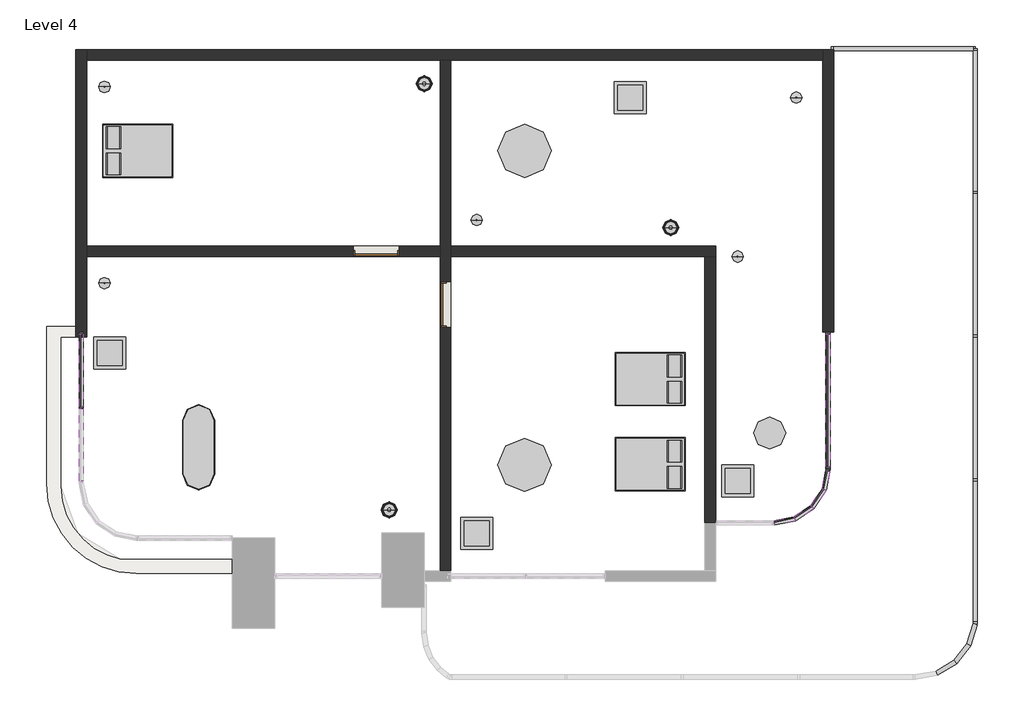
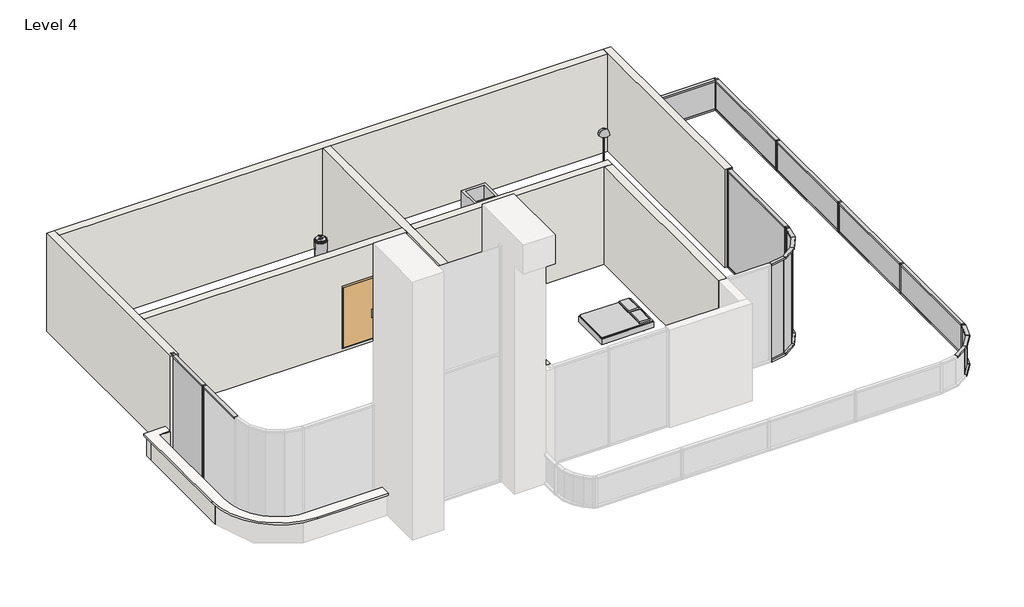
# One storey, part 2 of 2: 40 members, 13 plates, 9 walls, 7 furniture elements, 7 light fixtures, 4 geographic elements, 3 proxies, 2 doors, 1 slab.
"""IFC4 building model written with IfcOpenShell, lengths in millimetres."""

from ifc_helpers import new_model, si_unit, point, frame, frame_2d, origin, place, context, project, spatial, polyline, circle_curve, trimmed, segment, composite_curve, outline, extrude, faceted_brep, transform, mapped, element, save
from components import recycle_bin_round_recycle_bin_round_6e7ed866, door_bb6275b8, furniture_1d2926bd, furniture_e05f6f82, furniture_720490b2, furniture_905aceb5, geographic_element_4c884dac, floor_lamp_hemispheric_100w_120v_bd9db648, table_lamp_standard_100w_120v_6e8cd8b1, member_e5c989f4, member_5be86ab4, member_2115025b, member_820ab859, member_6051e8ad, member_ad26f02d, member_4ff03cd1, member_efc2c738, member_55924089, member_20b53a5f, member_9703a30f, member_ec2bec36, member_2b49869a, member_75074519, member_fe018dc2, member_83685764, member_73d0c9ee, system_panel_glazed_319e86f2, system_panel_glazed_5d8041e7, system_panel_glazed_56e4e121, system_panel_glazed_16a45962, system_panel_glazed_93b9a344, system_panel_glazed_b0cc1a2f, system_panel_glazed_8d4a2524, system_panel_glazed_b9e36109

model = new_model("IFC4")

# Units and contexts
model_context = context("Model", 3, world=origin())
ifc_project = project(units=[si_unit("LENGTHUNIT", "METRE", prefix="MILLI")], contexts=[model_context])

# Site, building, storey
site = spatial("IfcSite", under=ifc_project)
building = spatial("IfcBuilding", under=site)
storey = spatial("IfcBuildingStorey", under=building, Name="Level 4", Elevation=6096.0)

# Proxies
placement = place(None, origin())
recycle_bin_round_recycle_bin_round_shape = recycle_bin_round_recycle_bin_round_6e7ed866(model_context)
element("IfcBuildingElementProxy", 1, Name="Recycle Bin-Round : Recycle Bin-Round", ObjectType="Recycle Bin-Round : Recycle Bin-Round", at=placement, inside=storey, context=model_context, shape_type="MappedRepresentation", body=[
    mapped(recycle_bin_round_recycle_bin_round_shape, transform((-7920.936879, -2221.8562261, 6096.0), x_axis=(1.0, 0.0, 0.0), y_axis=(0.0, 1.0, 0.0), z_axis=(0.0, 0.0, 1.0))),
])
element("IfcBuildingElementProxy", 2, Name="Recycle Bin-Round : Recycle Bin-Round", ObjectType="Recycle Bin-Round : Recycle Bin-Round", at=placement, inside=storey, context=model_context, shape_type="MappedRepresentation", body=[
    mapped(recycle_bin_round_recycle_bin_round_shape, transform((-6917.636879, 9970.1437739, 6096.0), x_axis=(1.0, 0.0, 0.0), y_axis=(0.0, 1.0, 0.0), z_axis=(0.0, 0.0, 1.0))),
])
element("IfcBuildingElementProxy", 3, Name="Recycle Bin-Round : Recycle Bin-Round", ObjectType="Recycle Bin-Round : Recycle Bin-Round", at=placement, inside=storey, context=model_context, shape_type="MappedRepresentation", body=[
    mapped(recycle_bin_round_recycle_bin_round_shape, transform((130.863121, 5855.3437739, 6096.0), x_axis=(1.0, 0.0, 0.0), y_axis=(0.0, 1.0, 0.0), z_axis=(0.0, 0.0, 1.0))),
])

# Doors
door_shape = door_bb6275b8(model_context)
element("IfcDoor", 4, ObjectType="Door-Passage-Single-Flush-Dbl_Acting : 48\" x 96\"", at=placement, inside=storey, context=model_context, shape_type="MappedRepresentation", body=[
    mapped(door_shape, transform((-8289.236879, 5183.9591958, 6096.0), x_axis=(-1.0, 0.0, 0.0), y_axis=(0.0, -1.0, 0.0), z_axis=(0.0, 0.0, 1.0))),
])
element("IfcDoor", 5, ObjectType="Door-Passage-Single-Flush-Dbl_Acting : 48\" x 96\"", at=placement, inside=storey, context=model_context, shape_type="MappedRepresentation", body=[
    mapped(door_shape, transform((-6301.686879, 3653.6091958, 6096.0), x_axis=(0.0, 1.0, 0.0), y_axis=(-1.0, 0.0, 0.0), z_axis=(0.0, 0.0, 1.0))),
])

# Furniture
furniture_shape = furniture_1d2926bd(model_context)
element("IfcFurniture", 6, ObjectType="Bed-Box : Queen 60\" x 79\"", at=placement, inside=storey, context=model_context, shape_type="MappedRepresentation", body=[
    mapped(furniture_shape, transform((-15345.945017, 7713.2913149, 6096.0), x_axis=(0.0, 1.0000000000000002, 0.0), y_axis=(-1.0000000000000002, 0.0, 0.0), z_axis=(0.0, 0.0, 1.0))),
])
element("IfcFurniture", 7, ObjectType="Bed-Box : Queen 60\" x 79\"", at=placement, inside=storey, context=model_context, shape_type="MappedRepresentation", body=[
    mapped(furniture_shape, transform((-218.9073708, -579.2383452, 6096.0), x_axis=(0.0, -1.0, 0.0), y_axis=(1.0, 0.0, 0.0), z_axis=(0.0, 0.0, 1.0))),
])
element("IfcFurniture", 8, ObjectType="Bed-Box : Queen 60\" x 79\"", at=placement, inside=storey, context=model_context, shape_type="MappedRepresentation", body=[
    mapped(furniture_shape, transform((-218.9073708, 1859.1616548, 6096.0), x_axis=(0.0, -1.0, 0.0), y_axis=(1.0, 0.0, 0.0), z_axis=(0.0, 0.0, 1.0))),
])
furniture_2_shape = furniture_e05f6f82(model_context)
element("IfcFurniture", 9, ObjectType="Table-Dining Oval : 36\" x 96\" Glass Top", at=placement, inside=storey, context=model_context, shape_type="MappedRepresentation", body=[
    mapped(furniture_2_shape, transform((-13727.1545191, -29.9659461, 6096.0), x_axis=(0.0, 1.0000000000000002, 0.0), y_axis=(-1.0000000000000002, 0.0, 0.0), z_axis=(0.0, 0.0, 1.0))),
])
furniture_3_shape = furniture_720490b2(model_context)
element("IfcFurniture", 10, ObjectType="Table-Dining Round : 60\" Diameter", at=placement, inside=storey, context=model_context, shape_type="MappedRepresentation", body=[
    mapped(furniture_3_shape, transform((-4151.1188462, -754.2775376, 6096.0), x_axis=(1.0, 0.0, 0.0), y_axis=(0.0, 1.0, 0.0), z_axis=(0.0, 0.0, 1.0))),
])
element("IfcFurniture", 11, ObjectType="Table-Dining Round : 60\" Diameter", at=placement, inside=storey, context=model_context, shape_type="MappedRepresentation", body=[
    mapped(furniture_3_shape, transform((-4151.1188462, 8237.3224624, 6096.0), x_axis=(1.0, 0.0, 0.0), y_axis=(0.0, 1.0, 0.0), z_axis=(0.0, 0.0, 1.0))),
])
furniture_4_shape = furniture_905aceb5(model_context)
element("IfcFurniture", 12, ObjectType="Table-Dining Round w Chairs : 36\" Diameter", at=placement, inside=storey, context=model_context, shape_type="MappedRepresentation", body=[
    mapped(furniture_4_shape, transform((2855.1330373, 160.1224624, 6096.0), x_axis=(1.0, 0.0, 0.0), y_axis=(0.0, 1.0, 0.0), z_axis=(0.0, 0.0, 1.0))),
])

# Geographic elements
geographic_element_shape = geographic_element_4c884dac(model_context)
element("IfcGeographicElement", 13, ObjectType="Planter : 36\" x 36\"", at=placement, inside=storey, context=model_context, shape_type="MappedRepresentation", body=[
    mapped(geographic_element_shape, transform((2044.4150045, -1396.3562261, 6096.0), x_axis=(1.0, 0.0, 0.0), y_axis=(0.0, 1.0, 0.0), z_axis=(0.0, 0.0, 1.0))),
])
element("IfcGeographicElement", 14, ObjectType="Planter : 36\" x 36\"", at=placement, inside=storey, context=model_context, shape_type="MappedRepresentation", body=[
    mapped(geographic_element_shape, transform((-5419.036879, -2899.5908042, 6096.0), x_axis=(1.0, 0.0, 0.0), y_axis=(0.0, 1.0, 0.0), z_axis=(0.0, 0.0, 1.0))),
])
element("IfcGeographicElement", 15, ObjectType="Planter : 36\" x 36\"", at=placement, inside=storey, context=model_context, shape_type="MappedRepresentation", body=[
    mapped(geographic_element_shape, transform((-15909.236879, 2261.2437739, 6096.0), x_axis=(1.0, 0.0, 0.0), y_axis=(0.0, 1.0, 0.0), z_axis=(0.0, 0.0, 1.0))),
])
element("IfcGeographicElement", 16, ObjectType="Planter : 36\" x 36\"", at=placement, inside=storey, context=model_context, shape_type="MappedRepresentation", body=[
    mapped(geographic_element_shape, transform((-1024.836879, 9576.4437739, 6096.0), x_axis=(1.0, 0.0, 0.0), y_axis=(0.0, 1.0, 0.0), z_axis=(0.0, 0.0, 1.0))),
])

# Light fixtures
floor_lamp_hemispheric_100w_120v_shape = floor_lamp_hemispheric_100w_120v_bd9db648(model_context)
element("IfcLightFixture", 17, ObjectType="Floor Lamp - Hemispheric : 100W - 120V", at=placement, inside=storey, context=model_context, shape_type="MappedRepresentation", body=[
    mapped(floor_lamp_hemispheric_100w_120v_shape, transform((-16061.636879, 4263.2091958, 6096.0), x_axis=(1.0, 0.0, 0.0), y_axis=(0.0, 1.0, 0.0), z_axis=(0.0, 0.0, 1.0))),
])
element("IfcLightFixture", 18, ObjectType="Floor Lamp - Hemispheric : 100W - 120V", at=placement, inside=storey, context=model_context, shape_type="MappedRepresentation", body=[
    mapped(floor_lamp_hemispheric_100w_120v_shape, transform((-16061.636879, 9881.2437739, 6096.0), x_axis=(1.0, 0.0, 0.0), y_axis=(0.0, 1.0, 0.0), z_axis=(0.0, 0.0, 1.0))),
])
element("IfcLightFixture", 19, ObjectType="Floor Lamp - Hemispheric : 100W - 120V", at=placement, inside=storey, context=model_context, shape_type="MappedRepresentation", body=[
    mapped(floor_lamp_hemispheric_100w_120v_shape, transform((3720.8150045, 9576.4437739, 6096.0), x_axis=(1.0, 0.0, 0.0), y_axis=(0.0, 1.0, 0.0), z_axis=(0.0, 0.0, 1.0))),
])
element("IfcLightFixture", 20, ObjectType="Floor Lamp - Hemispheric : 100W - 120V", at=placement, inside=storey, context=model_context, shape_type="MappedRepresentation", body=[
    mapped(floor_lamp_hemispheric_100w_120v_shape, transform((2044.4150045, 5025.2091958, 6096.0), x_axis=(1.0, 0.0, 0.0), y_axis=(0.0, 1.0, 0.0), z_axis=(0.0, 0.0, 1.0))),
])
element("IfcLightFixture", 21, ObjectType="Floor Lamp - Hemispheric : 100W - 120V", at=placement, inside=storey, context=model_context, shape_type="MappedRepresentation", body=[
    mapped(floor_lamp_hemispheric_100w_120v_shape, transform((-5419.036879, 6071.2437739, 6096.0), x_axis=(1.0, 0.0, 0.0), y_axis=(0.0, 1.0, 0.0), z_axis=(0.0, 0.0, 1.0))),
])
table_lamp_standard_100w_120v_shape = table_lamp_standard_100w_120v_6e8cd8b1(model_context)
element("IfcLightFixture", 22, ObjectType="Table Lamp - Standard : 100W - 120V", at=placement, inside=storey, context=model_context, shape_type="MappedRepresentation", body=[
    mapped(table_lamp_standard_100w_120v_shape, transform((-4047.436879, -939.1562261, 6096.0), x_axis=(1.0, 0.0, 0.0), y_axis=(0.0, 1.0, 0.0), z_axis=(0.0, 0.0, 1.0))),
])
element("IfcLightFixture", 23, ObjectType="Table Lamp - Standard : 100W - 120V", at=placement, inside=storey, context=model_context, shape_type="MappedRepresentation", body=[
    mapped(table_lamp_standard_100w_120v_shape, transform((-4047.436879, 8052.4437739, 6096.0), x_axis=(1.0, 0.0, 0.0), y_axis=(0.0, 1.0, 0.0), z_axis=(0.0, 0.0, 1.0))),
])

# Members
member_shape = member_e5c989f4(model_context)
element("IfcMember", 24, ObjectType="Rectangular Mullion : 2.5\" x 5\" rectangular", at=placement, inside=storey, context=model_context, shape_type="MappedRepresentation", body=[
    mapped(member_shape, transform((-16724.4155088, 709.8310564, 5994.4), x_axis=(0.0, 1.0, 0.0), y_axis=(1.0, 0.0, 0.0), z_axis=(0.0, 0.0, -1.0))),
])
member_2_shape = member_5be86ab4(model_context)
element("IfcMember", 25, ObjectType="Rectangular Mullion : 2.5\" x 5\" rectangular", at=placement, inside=storey, context=model_context, shape_type="MappedRepresentation", body=[
    mapped(member_2_shape, transform((4635.2150045, -1049.5389207, 5994.4), x_axis=(0.19509032201613002, 0.9807852804032301, 0.0), y_axis=(0.9807852804032301, -0.19509032201613002, 0.0), z_axis=(0.0, 0.0, -1.0))),
])
element("IfcMember", 26, ObjectType="Rectangular Mullion : 2.5\" x 5\" rectangular", at=placement, inside=storey, context=model_context, shape_type="MappedRepresentation", body=[
    mapped(member_2_shape, transform((4635.2150045, 2870.8437739, 5994.4), x_axis=(0.0, 1.0, 0.0), y_axis=(1.0, 0.0, 0.0), z_axis=(0.0, 0.0, -1.0))),
])
element("IfcMember", 27, ObjectType="Rectangular Mullion : 2.5\" x 5\" rectangular", at=placement, inside=storey, context=model_context, shape_type="MappedRepresentation", body=[
    mapped(member_2_shape, transform((-16724.4155088, 2870.8437739, 5994.4), x_axis=(0.0, 1.0, 0.0), y_axis=(1.0, 0.0, 0.0), z_axis=(0.0, 0.0, -1.0))),
])
element("IfcMember", 28, ObjectType="Rectangular Mullion : 2.5\" x 5\" rectangular", at=placement, inside=storey, context=model_context, shape_type="MappedRepresentation", body=[
    mapped(member_2_shape, transform((4635.2150045, -1049.5389207, 9956.8), x_axis=(0.0, -1.0, 0.0), y_axis=(1.0, 0.0, 0.0), z_axis=(0.0, 0.0, 1.0))),
])
member_3_shape = member_2115025b(model_context)
element("IfcMember", 29, ObjectType="Rectangular Mullion : 2.5\" x 5\" rectangular", at=placement, inside=storey, context=model_context, shape_type="MappedRepresentation", body=[
    mapped(member_3_shape, transform((4635.2150045, 2807.3437739, 9956.8), x_axis=(0.0, 0.0, 1.0), y_axis=(1.0, 0.0, 0.0), z_axis=(0.0, 1.0, 0.0))),
])
element("IfcMember", 30, ObjectType="Rectangular Mullion : 2.5\" x 5\" rectangular", at=placement, inside=storey, context=model_context, shape_type="MappedRepresentation", body=[
    mapped(member_3_shape, transform((4635.2150045, -986.0389207, 5994.4), x_axis=(0.0, 0.0, -1.0), y_axis=(1.0, 0.0, 0.0), z_axis=(0.0, -1.0, 0.0))),
])
member_4_shape = member_820ab859(model_context)
element("IfcMember", 31, ObjectType="Rectangular Mullion : 2.5\" x 5\" rectangular", at=placement, inside=storey, context=model_context, shape_type="MappedRepresentation", body=[
    mapped(member_4_shape, transform((-16724.4155088, 2807.3437739, 9956.8), x_axis=(0.0, 0.0, 1.0), y_axis=(1.0, 0.0, 0.0), z_axis=(0.0, 1.0, 0.0))),
])
element("IfcMember", 32, ObjectType="Rectangular Mullion : 2.5\" x 5\" rectangular", at=placement, inside=storey, context=model_context, shape_type="MappedRepresentation", body=[
    mapped(member_4_shape, transform((-16724.4155088, 678.0810564, 9956.8), x_axis=(0.0, 0.0, 1.0), y_axis=(1.0, 0.0, 0.0), z_axis=(0.0, 1.0, 0.0))),
])
element("IfcMember", 33, ObjectType="Rectangular Mullion : 2.5\" x 5\" rectangular", at=placement, inside=storey, context=model_context, shape_type="MappedRepresentation", body=[
    mapped(member_4_shape, transform((-16724.4155088, 741.5810564, 5994.4), x_axis=(0.0, 0.0, -1.0), y_axis=(1.0, 0.0, 0.0), z_axis=(0.0, -1.0, 0.0))),
])
member_5_shape = member_6051e8ad(model_context)
element("IfcMember", 34, ObjectType="Rectangular Mullion : 2.5\" x 5\" rectangular", at=placement, inside=storey, context=model_context, shape_type="MappedRepresentation", body=[
    mapped(member_5_shape, transform((3089.963121, -2594.7908042, 5994.4), x_axis=(0.0, 0.0, -1.0), y_axis=(0.19509032201612592, -0.9807852804032309, 0.0), z_axis=(-0.9807852804032309, -0.19509032201612592, 0.0))),
])
member_6_shape = member_ad26f02d(model_context)
element("IfcMember", 35, ObjectType="Rectangular Mullion : 2.5\" x 5\" rectangular", at=placement, inside=storey, context=model_context, shape_type="MappedRepresentation", body=[
    mapped(member_6_shape, transform((3681.3054157, -2477.1655084, 9956.8), x_axis=(0.0, 0.0, 1.0), y_axis=(0.19509032201612592, -0.9807852804032309, 0.0), z_axis=(0.9807852804032309, 0.19509032201612592, 0.0))),
])
member_7_shape = member_4ff03cd1(model_context)
element("IfcMember", 36, ObjectType="Rectangular Mullion : 2.5\" x 5\" rectangular", at=placement, inside=storey, context=model_context, shape_type="MappedRepresentation", body=[
    mapped(member_7_shape, transform((4182.6212065, -2142.1970062, 9956.8), x_axis=(0.0, 0.0, 1.0), y_axis=(0.5555702330196008, -0.8314696123025462, 0.0), z_axis=(0.8314696123025462, 0.5555702330196008, 0.0))),
])
element("IfcMember", 37, ObjectType="Rectangular Mullion : 2.5\" x 5\" rectangular", at=placement, inside=storey, context=model_context, shape_type="MappedRepresentation", body=[
    mapped(member_7_shape, transform((3681.3054157, -2477.1655084, 5994.4), x_axis=(0.0, 0.0, -1.0), y_axis=(0.5555702330196008, -0.8314696123025462, 0.0), z_axis=(-0.8314696123025462, -0.5555702330196008, 0.0))),
])
member_8_shape = member_efc2c738(model_context)
element("IfcMember", 38, ObjectType="Rectangular Mullion : 2.5\" x 5\" rectangular", at=placement, inside=storey, context=model_context, shape_type="MappedRepresentation", body=[
    mapped(member_8_shape, transform((4622.826769, -1111.818786, 9956.8), x_axis=(0.0, 0.0, 1.0), y_axis=(0.9807852804032301, -0.19509032201613, 0.0), z_axis=(0.19509032201612997, 0.98078528040323, 0.0))),
])
element("IfcMember", 39, ObjectType="Rectangular Mullion : 2.5\" x 5\" rectangular", at=placement, inside=storey, context=model_context, shape_type="MappedRepresentation", body=[
    mapped(member_7_shape, transform((4182.6212065, -2142.1970062, 5994.4), x_axis=(0.0, 0.0, -1.0), y_axis=(0.831469612302544, -0.5555702330196041, 0.0), z_axis=(-0.5555702330196041, -0.831469612302544, 0.0))),
])
element("IfcMember", 40, ObjectType="Rectangular Mullion : 2.5\" x 5\" rectangular", at=placement, inside=storey, context=model_context, shape_type="MappedRepresentation", body=[
    mapped(member_7_shape, transform((4517.5897087, -1640.8812154, 9956.8), x_axis=(0.0, 0.0, 1.0), y_axis=(0.831469612302544, -0.5555702330196041, 0.0), z_axis=(0.5555702330196041, 0.831469612302544, 0.0))),
])
member_9_shape = member_55924089(model_context)
element("IfcMember", 41, ObjectType="Rectangular Mullion : 2.5\" x 5\" rectangular", at=placement, inside=storey, context=model_context, shape_type="MappedRepresentation", body=[
    mapped(member_9_shape, transform((4517.5897087, -1640.8812154, 5994.4), x_axis=(0.0, 0.0, -1.0), y_axis=(0.9807852804032301, -0.19509032201613008, 0.0), z_axis=(-0.19509032201613008, -0.9807852804032301, 0.0))),
])
member_10_shape = member_20b53a5f(model_context)
element("IfcMember", 42, ObjectType="Rectangular Mullion : 2.5\" x 5\" rectangular", at=placement, inside=storey, context=model_context, shape_type="MappedRepresentation", body=[
    mapped(member_10_shape, transform((8839.2, 10909.3, 7213.6), x_axis=(0.0, 0.0, 1.0), y_axis=(1.0, 0.0, 0.0), z_axis=(0.0, 1.0, 0.0))),
])
element("IfcMember", 43, ObjectType="Rectangular Mullion : 2.5\" x 5\" rectangular", at=placement, inside=storey, context=model_context, shape_type="MappedRepresentation", body=[
    mapped(member_10_shape, transform((8839.2, -1403.35, 7213.6), x_axis=(0.0, 0.0, 1.0), y_axis=(1.0, 0.0, 0.0), z_axis=(0.0, 1.0, 0.0))),
])
member_11_shape = member_9703a30f(model_context)
element("IfcMember", 44, ObjectType="Rectangular Mullion : 2.5\" x 5\" rectangular", at=placement, inside=storey, context=model_context, shape_type="MappedRepresentation", body=[
    mapped(member_11_shape, transform((8839.2, 2711.45, 7213.6), x_axis=(0.0, 0.0, 1.0), y_axis=(1.0, 0.0, 0.0), z_axis=(0.0, 1.0, 0.0))),
])
element("IfcMember", 45, ObjectType="Rectangular Mullion : 2.5\" x 5\" rectangular", at=placement, inside=storey, context=model_context, shape_type="MappedRepresentation", body=[
    mapped(member_11_shape, transform((8839.2, 6826.25, 7213.6), x_axis=(0.0, 0.0, 1.0), y_axis=(1.0, 0.0, 0.0), z_axis=(0.0, 1.0, 0.0))),
])
element("IfcMember", 46, ObjectType="Rectangular Mullion : 2.5\" x 5\" rectangular", at=placement, inside=storey, context=model_context, shape_type="MappedRepresentation", body=[
    mapped(member_10_shape, transform((8839.2, -5422.9, 5994.4), x_axis=(0.0, 0.0, -1.0), y_axis=(1.0, 0.0, 0.0), z_axis=(0.0, -1.0, 0.0))),
])
element("IfcMember", 47, ObjectType="Rectangular Mullion : 2.5\" x 5\" rectangular", at=placement, inside=storey, context=model_context, shape_type="MappedRepresentation", body=[
    mapped(member_10_shape, transform((8839.2, 6889.75, 5994.4), x_axis=(0.0, 0.0, -1.0), y_axis=(1.0, 0.0, 0.0), z_axis=(0.0, -1.0, 0.0))),
])
element("IfcMember", 48, ObjectType="Rectangular Mullion : 2.5\" x 5\" rectangular", at=placement, inside=storey, context=model_context, shape_type="MappedRepresentation", body=[
    mapped(member_11_shape, transform((8839.2, -1339.85, 5994.4), x_axis=(0.0, 0.0, -1.0), y_axis=(1.0, 0.0, 0.0), z_axis=(0.0, -1.0, 0.0))),
])
element("IfcMember", 49, ObjectType="Rectangular Mullion : 2.5\" x 5\" rectangular", at=placement, inside=storey, context=model_context, shape_type="MappedRepresentation", body=[
    mapped(member_11_shape, transform((8839.2, 2774.95, 5994.4), x_axis=(0.0, 0.0, -1.0), y_axis=(1.0, 0.0, 0.0), z_axis=(0.0, -1.0, 0.0))),
])
member_12_shape = member_ec2bec36(model_context)
element("IfcMember", 50, ObjectType="Rectangular Mullion : 2.5\" x 5\" rectangular", at=placement, inside=storey, context=model_context, shape_type="MappedRepresentation", body=[
    mapped(member_12_shape, transform((4787.9, 10972.8, 7213.6), x_axis=(0.0, 0.0, 1.0), y_axis=(0.0, 1.0, 0.0), z_axis=(-1.0, 0.0, 0.0))),
])
element("IfcMember", 51, ObjectType="Rectangular Mullion : 2.5\" x 5\" rectangular", at=placement, inside=storey, context=model_context, shape_type="MappedRepresentation", body=[
    mapped(member_12_shape, transform((8775.7, 10972.8, 5994.4), x_axis=(0.0, 0.0, -1.0), y_axis=(0.0, 1.0, 0.0), z_axis=(1.0, 0.0, 0.0))),
])
member_13_shape = member_2b49869a(model_context)
element("IfcMember", 52, ObjectType="Rectangular Mullion : 2.5\" x 5\" rectangular", at=placement, inside=storey, context=model_context, shape_type="MappedRepresentation", body=[
    mapped(member_13_shape, transform((8839.2, -1371.6, 5994.4), x_axis=(0.0, 1.0, 0.0), y_axis=(1.0, 0.0, 0.0), z_axis=(0.0, 0.0, -1.0))),
])
element("IfcMember", 53, ObjectType="Rectangular Mullion : 2.5\" x 5\" rectangular", at=placement, inside=storey, context=model_context, shape_type="MappedRepresentation", body=[
    mapped(member_13_shape, transform((8839.2, 2743.2, 5994.4), x_axis=(0.0, 1.0, 0.0), y_axis=(1.0, 0.0, 0.0), z_axis=(0.0, 0.0, -1.0))),
])
element("IfcMember", 54, ObjectType="Rectangular Mullion : 2.5\" x 5\" rectangular", at=placement, inside=storey, context=model_context, shape_type="MappedRepresentation", body=[
    mapped(member_13_shape, transform((8839.2, 6858.0, 5994.4), x_axis=(0.0, 1.0, 0.0), y_axis=(1.0, 0.0, 0.0), z_axis=(0.0, 0.0, -1.0))),
])
member_14_shape = member_75074519(model_context)
element("IfcMember", 55, ObjectType="Rectangular Mullion : 2.5\" x 5\" rectangular", at=placement, inside=storey, context=model_context, shape_type="MappedRepresentation", body=[
    mapped(member_14_shape, transform((8839.2, 10972.8, 5994.4), x_axis=(0.0, 1.0, 0.0), y_axis=(1.0, 0.0, 0.0), z_axis=(0.0, 0.0, -1.0))),
])
element("IfcMember", 56, ObjectType="Rectangular Mullion : 2.5\" x 5\" rectangular", at=placement, inside=storey, context=model_context, shape_type="MappedRepresentation", body=[
    mapped(member_14_shape, transform((4724.4, 10972.8, 5994.4), x_axis=(-1.0, 0.0, 0.0), y_axis=(0.0, 1.0, 0.0), z_axis=(0.0, 0.0, -1.0))),
])
element("IfcMember", 57, ObjectType="Rectangular Mullion : 2.5\" x 5\" rectangular", at=placement, inside=storey, context=model_context, shape_type="MappedRepresentation", body=[
    mapped(member_14_shape, transform((8839.2, -5486.4, 7213.6), x_axis=(0.0, -1.0, 0.0), y_axis=(1.0, 0.0, 0.0), z_axis=(0.0, 0.0, 1.0))),
])
element("IfcMember", 58, ObjectType="Rectangular Mullion : 2.5\" x 5\" rectangular", at=placement, inside=storey, context=model_context, shape_type="MappedRepresentation", body=[
    mapped(member_14_shape, transform((8839.2, 10972.8, 7213.6), x_axis=(1.0, 0.0, 0.0), y_axis=(0.0, 1.0, 0.0), z_axis=(0.0, 0.0, 1.0))),
])
member_15_shape = member_fe018dc2(model_context)
element("IfcMember", 59, ObjectType="Rectangular Mullion : 2.5\" x 5\" rectangular", at=placement, inside=storey, context=model_context, shape_type="MappedRepresentation", body=[
    mapped(member_15_shape, transform((8263.7156594, -6574.9310806, 5994.4), x_axis=(0.0, 0.0, -1.0), y_axis=(0.7856364667820415, -0.6186884046612077, 0.0), z_axis=(-0.6186884046612077, -0.7856364667820415, 0.0))),
])
element("IfcMember", 60, ObjectType="Rectangular Mullion : 2.5\" x 5\" rectangular", at=placement, inside=storey, context=model_context, shape_type="MappedRepresentation", body=[
    mapped(member_15_shape, transform((8650.9164441, -6083.2472958, 7213.6), x_axis=(0.0, 0.0, 1.0), y_axis=(0.7856364667820415, -0.6186884046612077, 0.0), z_axis=(0.6186884046612077, 0.7856364667820415, 0.0))),
])
element("IfcMember", 61, ObjectType="Rectangular Mullion : 2.5\" x 5\" rectangular", at=placement, inside=storey, context=model_context, shape_type="MappedRepresentation", body=[
    mapped(member_15_shape, transform((8263.7156594, -6574.9310806, 7213.6), x_axis=(0.0, 0.0, 1.0), y_axis=(0.5160512694614295, -0.856557696414694, 0.0), z_axis=(0.8565576964146939, 0.5160512694614294, 0.0))),
])
member_16_shape = member_83685764(model_context)
element("IfcMember", 62, ObjectType="Rectangular Mullion : 2.5\" x 5\" rectangular", at=placement, inside=storey, context=model_context, shape_type="MappedRepresentation", body=[
    mapped(member_16_shape, transform((8839.2, -5486.4, 7213.6), x_axis=(0.0, 0.0, 1.0), y_axis=(0.9536718825126238, -0.30084870035422845, 0.0), z_axis=(0.30084870035422845, 0.9536718825126238, 0.0))),
])
member_17_shape = member_73d0c9ee(model_context)
element("IfcMember", 63, ObjectType="Rectangular Mullion : 2.5\" x 5\" rectangular", at=placement, inside=storey, context=model_context, shape_type="MappedRepresentation", body=[
    mapped(member_17_shape, transform((8650.9164441, -6083.2472958, 5994.4), x_axis=(0.0, 0.0, -1.0), y_axis=(0.9536718825126238, -0.30084870035422845, 0.0), z_axis=(-0.30084870035422845, -0.9536718825126238, 0.0))),
])

# Plates
system_panel_glazed_shape = system_panel_glazed_319e86f2(model_context)
element("IfcPlate", 64, ObjectType="System Panel : Glazed", at=placement, inside=storey, context=model_context, shape_type="MappedRepresentation", body=[
    mapped(system_panel_glazed_shape, transform((4635.2150045, 910.6524266, 6057.9), x_axis=(0.0, 1.0, 0.0), y_axis=(-1.0, 0.0, 0.0), z_axis=(0.0, 0.0, 1.0))),
])
system_panel_glazed_2_shape = system_panel_glazed_5d8041e7(model_context)
element("IfcPlate", 65, ObjectType="System Panel : Glazed", at=placement, inside=storey, context=model_context, shape_type="MappedRepresentation", body=[
    mapped(system_panel_glazed_2_shape, transform((-16724.4155088, 1774.4624152, 6057.9), x_axis=(0.0, 1.0, 0.0), y_axis=(-1.0, 0.0, 0.0), z_axis=(0.0, 0.0, 1.0))),
])
system_panel_glazed_3_shape = system_panel_glazed_56e4e121(model_context)
element("IfcPlate", 66, ObjectType="System Panel : Glazed", at=placement, inside=storey, context=model_context, shape_type="MappedRepresentation", body=[
    mapped(system_panel_glazed_3_shape, transform((3385.6342684, -2535.9781563, 6057.9), x_axis=(0.9807852804032309, 0.1950903220161259, 0.0), y_axis=(-0.1950903220161259, 0.9807852804032309, 0.0), z_axis=(0.0, 0.0, 1.0))),
])
element("IfcPlate", 67, ObjectType="System Panel : Glazed", at=placement, inside=storey, context=model_context, shape_type="MappedRepresentation", body=[
    mapped(system_panel_glazed_3_shape, transform((4350.1054576, -1891.5391108, 6057.9), x_axis=(0.5555702330196041, 0.831469612302544, 0.0), y_axis=(-0.831469612302544, 0.5555702330196041, 0.0), z_axis=(0.0, 0.0, 1.0))),
])
element("IfcPlate", 68, ObjectType="System Panel : Glazed", at=placement, inside=storey, context=model_context, shape_type="MappedRepresentation", body=[
    mapped(system_panel_glazed_3_shape, transform((3931.9633111, -2309.6812573, 6057.9), x_axis=(0.8314696123025462, 0.5555702330196008, 0.0), y_axis=(-0.5555702330196008, 0.8314696123025462, 0.0), z_axis=(0.0, 0.0, 1.0))),
])
system_panel_glazed_4_shape = system_panel_glazed_16a45962(model_context)
element("IfcPlate", 69, ObjectType="System Panel : Glazed", at=placement, inside=storey, context=model_context, shape_type="MappedRepresentation", body=[
    mapped(system_panel_glazed_4_shape, transform((4570.2082389, -1376.3500007, 6057.9), x_axis=(0.19509032201613002, 0.9807852804032301, 0.0), y_axis=(-0.9807852804032301, 0.19509032201613002, 0.0), z_axis=(0.0, 0.0, 1.0))),
])
system_panel_glazed_5_shape = system_panel_glazed_93b9a344(model_context)
element("IfcPlate", 70, ObjectType="System Panel : Glazed", at=placement, inside=storey, context=model_context, shape_type="MappedRepresentation", body=[
    mapped(system_panel_glazed_5_shape, transform((8839.2, -3413.125, 6057.9), x_axis=(0.0, 1.0, 0.0), y_axis=(-1.0, 0.0, 0.0), z_axis=(0.0, 0.0, 1.0))),
])
element("IfcPlate", 71, ObjectType="System Panel : Glazed", at=placement, inside=storey, context=model_context, shape_type="MappedRepresentation", body=[
    mapped(system_panel_glazed_5_shape, transform((8839.2, 8899.525, 6057.9), x_axis=(0.0, 1.0, 0.0), y_axis=(-1.0, 0.0, 0.0), z_axis=(0.0, 0.0, 1.0))),
])
system_panel_glazed_6_shape = system_panel_glazed_b0cc1a2f(model_context)
element("IfcPlate", 72, ObjectType="System Panel : Glazed", at=placement, inside=storey, context=model_context, shape_type="MappedRepresentation", body=[
    mapped(system_panel_glazed_6_shape, transform((8839.2, 685.8, 6057.9), x_axis=(0.0, 1.0, 0.0), y_axis=(-1.0, 0.0, 0.0), z_axis=(0.0, 0.0, 1.0))),
])
element("IfcPlate", 73, ObjectType="System Panel : Glazed", at=placement, inside=storey, context=model_context, shape_type="MappedRepresentation", body=[
    mapped(system_panel_glazed_6_shape, transform((8839.2, 4800.6, 6057.9), x_axis=(0.0, 1.0, 0.0), y_axis=(-1.0, 0.0, 0.0), z_axis=(0.0, 0.0, 1.0))),
])
system_panel_glazed_7_shape = system_panel_glazed_8d4a2524(model_context)
element("IfcPlate", 74, ObjectType="System Panel : Glazed", at=placement, inside=storey, context=model_context, shape_type="MappedRepresentation", body=[
    mapped(system_panel_glazed_7_shape, transform((6781.8, 10972.8, 6057.9), x_axis=(-1.0, 0.0, 0.0), y_axis=(0.0, -1.0, 0.0), z_axis=(0.0, 0.0, 1.0))),
])
system_panel_glazed_8_shape = system_panel_glazed_b9e36109(model_context)
element("IfcPlate", 75, ObjectType="System Panel : Glazed", at=placement, inside=storey, context=model_context, shape_type="MappedRepresentation", body=[
    mapped(system_panel_glazed_8_shape, transform((8457.3160517, -6329.0891882, 6057.9), x_axis=(0.6186884046612077, 0.7856364667820415, 0.0), y_axis=(-0.7856364667820415, 0.6186884046612077, 0.0), z_axis=(0.0, 0.0, 1.0))),
])
element("IfcPlate", 76, ObjectType="System Panel : Glazed", at=placement, inside=storey, context=model_context, shape_type="MappedRepresentation", body=[
    mapped(system_panel_glazed_8_shape, transform((8745.058222, -5784.8236479, 6057.9), x_axis=(0.30084870035422845, 0.9536718825126238, 0.0), y_axis=(-0.9536718825126238, 0.30084870035422845, 0.0), z_axis=(0.0, 0.0, 1.0))),
])

# Slab
element("IfcSlab", 77, ObjectType="Generic - 3\"", at=placement, inside=storey, context=model_context, shape_type="SweptSolid", body=[
    extrude(outline(composite_curve([segment(polyline([(-17716.7849955, 3023.2437739), (-16876.8155088, 3023.2437739), (-16876.8155088, 2718.4437739), (-17310.3849955, 2718.4437739), (-17310.3849955, -1548.7562261)]), True, "CONTINUOUS"), segment(trimmed(circle_curve(frame_2d((-15181.4461231, -1548.7562261)), 2128.9388724), [point((-17310.3849955, -1548.7562261))], [point((-15599.7732735, -3636.1908042))], True, "CARTESIAN"), True, "CONTINUOUS"), segment(polyline([(-15599.7732735, -3636.1908042), (-12404.036879, -3636.1908042), (-12404.036879, -4044.3602909), (-15147.236879, -4044.3602909)]), True, "CONTINUOUS"), segment(trimmed(circle_curve(frame_2d((-15147.236879, -1474.8121743)), 2569.5481165), [point((-15147.236879, -4044.3602909))], [point((-17716.7849955, -1474.8121743))], False, "CARTESIAN"), True, "CONTINUOUS"), segment(polyline([(-17716.7849955, -1474.8121743), (-17716.7849955, 3023.2437739)]), True, "CONTINUOUS")], self_intersect=False)), frame((0.0, 0.0, 6858.0), z_axis=(0.0, 0.0, 1.0), x_axis=(1.0, 0.0, 0.0)), (0.0, 0.0, 1.0), 76.2),
])

# Walls
element("IfcWall", 78, ObjectType="Generic - 12\"", at=placement, inside=storey, context=model_context, shape_type="Brep", body=[
    faceted_brep([(4482.8150045, 10948.0437739, 5994.4), (4482.8150045, 10643.2437739, 5994.4), (4482.8150045, 2870.8437739, 5994.4), (4482.8150045, 2870.8437739, 9956.8), (4482.8150045, 10643.2437739, 9956.8), (4482.8150045, 10948.0437739, 9956.8), (4787.6150045, 10948.0437739, 5994.4), (4787.6150045, 10948.0437739, 9956.8), (4787.6150045, 2870.8437739, 9956.8), (4787.6150045, 2870.8437739, 5994.4)], [[[0, 1, 2, 3, 4, 5]], [[6, 7, 8, 9]], [[2, 1, 0, 6, 9]], [[3, 2, 9, 8]], [[5, 4, 3, 8, 7]], [[0, 5, 7, 6]]]),
])
element("IfcWall", 79, ObjectType="Generic - 12\"", at=placement, inside=storey, context=model_context, shape_type="Brep", body=[
    faceted_brep([(-16876.8155088, 10948.0437739, 5994.4), (-16876.8155088, 3023.2437739, 5994.4), (-16876.8155088, 2718.4437739, 5994.4), (-16876.8155088, 2718.4437739, 6908.8), (-16876.8155088, 2718.4437739, 9956.8), (-16876.8155088, 10948.0437739, 9956.8), (-16572.0155088, 10948.0437739, 5994.4), (-16572.0155088, 10948.0437739, 9956.8), (-16572.0155088, 10643.2437739, 9956.8), (-16572.0155088, 5330.0091958, 9956.8), (-16572.0155088, 5025.2091958, 9956.8), (-16572.0155088, 2718.4437739, 9956.8), (-16572.0155088, 2718.4437739, 5994.4), (-16572.0155088, 5025.2091958, 5994.4), (-16572.0155088, 5330.0091958, 5994.4), (-16572.0155088, 10643.2437739, 5994.4)], [[[0, 1, 2, 3, 4, 5]], [[6, 7, 8, 9, 10, 11, 12, 13, 14, 15]], [[2, 1, 0, 6, 15, 14, 13, 12]], [[5, 4, 11, 10, 9, 8, 7]], [[0, 5, 7, 6]], [[4, 3, 2, 12, 11]]]),
])
element("IfcWall", 80, ObjectType="Generic - 12\"", at=placement, inside=storey, context=model_context, shape_type="Brep", body=[
    faceted_brep([(-16572.0155088, 10643.2437739, 5994.4), (-6460.436879, 10643.2437739, 5994.4), (-6155.636879, 10643.2437739, 5994.4), (4482.8150045, 10643.2437739, 5994.4), (4482.8150045, 10643.2437739, 9956.8), (-6155.636879, 10643.2437739, 9956.8), (-6460.436879, 10643.2437739, 9956.8), (-16572.0155088, 10643.2437739, 9956.8), (-16572.0155088, 10948.0437739, 5994.4), (-16572.0155088, 10948.0437739, 9956.8), (4482.8150045, 10948.0437739, 9956.8), (4482.8150045, 10948.0437739, 5994.4)], [[[0, 1, 2, 3, 4, 5, 6, 7]], [[8, 9, 10, 11]], [[3, 2, 1, 0, 8, 11]], [[7, 6, 5, 4, 10, 9]], [[0, 7, 9, 8]], [[4, 3, 11, 10]]]),
])
element("IfcWall", 81, ObjectType="Generic - 12\"", at=placement, inside=storey, context=model_context, shape_type="Brep", body=[
    faceted_brep([(-16876.8155088, 3023.2437739, 5994.4), (-17615.1849955, 3023.2437739, 5994.4), (-17615.1849955, 3023.2437739, 6908.8), (-16876.8155088, 3023.2437739, 6908.8), (-16876.8155088, 2718.4437739, 5994.4), (-16876.8155088, 2718.4437739, 6908.8), (-17310.3849955, 2718.4437739, 6908.8), (-17615.1849955, 2718.4437739, 6908.8), (-17615.1849955, 2718.4437739, 5994.4), (-17310.3849955, 2718.4437739, 5994.4)], [[[0, 1, 2, 3]], [[4, 5, 6, 7, 8, 9]], [[1, 0, 4, 9, 8]], [[3, 2, 7, 6, 5]], [[0, 3, 5, 4]], [[2, 1, 8, 7]]]),
])
element("IfcWall", 82, ObjectType="Generic - 12\"", at=placement, inside=storey, context=model_context, shape_type="SweptSolid", body=[
    extrude(outline(polyline([(-17615.1849955, -1548.7562261), (-17615.1849955, 2718.4437739), (-17310.3849955, 2718.4437739), (-17310.3849955, -1548.7562261), (-17615.1849955, -1548.7562261)])), frame((0.0, 0.0, 5994.4), z_axis=(0.0, 0.0, 1.0), x_axis=(1.0, 0.0, 0.0)), (0.0, 0.0, 1.0), 914.4),
])
element("IfcWall", 83, ObjectType="Generic - 12\" yellow", at=placement, inside=storey, context=model_context, shape_type="Brep", body=[
    faceted_brep([(-6460.436879, 10643.2437739, 5994.4), (-6460.436879, 5330.0091958, 5994.4), (-6460.436879, 5025.2091958, 5994.4), (-6460.436879, -3966.3908042, 5994.4), (-6460.436879, -3966.3908042, 9956.8), (-6460.436879, 5025.2091958, 9956.8), (-6460.436879, 5330.0091958, 9956.8), (-6460.436879, 10643.2437739, 9956.8), (-6460.436879, 4314.0091958, 6096.0), (-6460.436879, 4314.0091958, 8636.0), (-6460.436879, 2993.2091958, 8636.0), (-6460.436879, 2993.2091958, 6096.0), (-6155.636879, 10643.2437739, 5994.4), (-6155.636879, 10643.2437739, 9956.8), (-6155.636879, 5330.0091958, 9956.8), (-6155.636879, 5025.2091958, 9956.8), (-6155.636879, -3966.3908042, 9956.8), (-6155.636879, -3966.3908042, 5994.4), (-6155.636879, 5025.2091958, 5994.4), (-6155.636879, 5330.0091958, 5994.4), (-6155.636879, 4314.0091958, 6096.0), (-6155.636879, 2993.2091958, 6096.0), (-6155.636879, 2993.2091958, 8636.0), (-6155.636879, 4314.0091958, 8636.0)], [[[0, 1, 2, 3, 4, 5, 6, 7], [8, 9, 10, 11]], [[12, 13, 14, 15, 16, 17, 18, 19], [20, 21, 22, 23]], [[3, 2, 1, 0, 12, 19, 18, 17]], [[7, 6, 5, 4, 16, 15, 14, 13]], [[4, 3, 17, 16]], [[0, 7, 13, 12]], [[9, 8, 20, 23]], [[10, 9, 23, 22]], [[11, 10, 22, 21]], [[8, 11, 21, 20]]]),
])
element("IfcWall", 84, ObjectType="Generic - 12\" yellow", at=placement, inside=storey, context=model_context, shape_type="Brep", body=[
    faceted_brep([(-6155.636879, 5025.2091958, 5994.4), (1108.763121, 5025.2091958, 5994.4), (1413.563121, 5025.2091958, 5994.4), (1413.563121, 5025.2091958, 9956.8), (1108.763121, 5025.2091958, 9956.8), (-6155.636879, 5025.2091958, 9956.8), (-6155.636879, 5330.0091958, 5994.4), (-6155.636879, 5330.0091958, 9956.8), (1413.563121, 5330.0091958, 9956.8), (1413.563121, 5330.0091958, 5994.4)], [[[0, 1, 2, 3, 4, 5]], [[6, 7, 8, 9]], [[2, 1, 0, 6, 9]], [[5, 4, 3, 8, 7]], [[0, 5, 7, 6]], [[3, 2, 9, 8]]]),
])
element("IfcWall", 85, ObjectType="Generic - 12\" yellow", at=placement, inside=storey, context=model_context, shape_type="SweptSolid", body=[
    extrude(outline(polyline([(1108.763121, -2594.7908042), (1108.763121, 5025.2091958), (1413.563121, 5025.2091958), (1413.563121, -2594.7908042), (1108.763121, -2594.7908042)])), frame((0.0, 0.0, 5994.4), z_axis=(0.0, 0.0, 1.0), x_axis=(1.0, 0.0, 0.0)), (0.0, 0.0, 1.0), 3962.4),
])
element("IfcWall", 86, ObjectType="Generic - 12\" yellow", at=placement, inside=storey, context=model_context, shape_type="SweptSolid", body=[
    extrude(outline(polyline([(5994.4, -6460.436879), (9956.8, -6460.436879), (9956.8, -16572.0155088), (5994.4, -16572.0155088), (5994.4, -6460.436879)]), holes=[polyline([(6096.0, -8949.636879), (8636.0, -8949.636879), (8636.0, -7628.836879), (6096.0, -7628.836879), (6096.0, -8949.636879)])]), frame((0.0, 5025.2091958, 0.0), z_axis=(0.0, 1.0, 0.0), x_axis=(0.0, 0.0, 1.0)), (0.0, 0.0, 1.0), 304.8),
])

save(model, "model.ifc")

# Revit data of these elements
# Type "Recycle Bin-Round : Recycle Bin-Round"
#   Default Elevation = 0
# Type "Door-Passage-Single-Flush-Dbl_Acting : 48\" x 96\""
#   Type Mark = "8"
#   Assembly Code = "B2030200"
#   Analytic Construction = "Wooden"
#   Thickness = 0' - 1 3/4"
#   Thermal Resistance (R) = 2.5876 (h·ft²·°F)/BTU
#   Swing Angle [instance default] = 45.00°
#   Strike Height = 3' - 4"
#   Rough Width [instance default] = 4' - 4"
#   Rough Height [instance default] = 8' - 4"
#   MF Opening Height [instance default] = 0' - 4"
#   MF Opening Width [instance default] = 0' - 4"
#   Inset Calculate [instance default] = 0' - 4"
#   Masonry Inset [instance default] = 0' - 1"
#   Height = 8' - 0"
#   Width = 4' - 0"
#   Heat Transfer Coefficient (U) = 0.3865 BTU/(h·ft²·°F)
#   Masonry Frame Depth = 0' - 5 3/4"
#   Masonry Frame [instance default] = yes
#   Function = 1
#   Dry Wall Frame [instance default] = no
#   Panel Material = Wood - Birch
#   Frame Material = Metal - Paint Finish - Grey
#   Door Handle Material = Aluminum
#   Visual Light Transmittance = 0
#   Solar Heat Gain Coefficient = 0
#   Wall Closure = (empty or 0)
# Type "Bed-Box : Queen 60\" x 79\""
#   Assembly Code = "E2020200"
#   Length = 6' - 7"
#   Width = 5' - 0"
#   Frame Material = Birch
#   Mattress Material = Linen, White
#   Default Elevation = 0
# Type "Table-Dining Oval : 36\" x 96\" Glass Top"
#   Assembly Code = "E2020200"
#   Length = 8' - 0"
#   Width = 3' - 0"
#   Base Material = Steel, Chrome Plated
#   Top Material = Glass - Clear, Grey
#   Default Elevation = 0
#   Description = (empty or 0)
# Type "Table-Dining Round : 60\" Diameter"
#   Assembly Code = "E2020200"
#   Diameter = 5' - 0"
#   Height = 2' - 6"
#   Base Material = Pine
#   Top Material = Laminate, Linen, Matte
#   Default Elevation = 0
# Type "Table-Dining Round w Chairs : 36\" Diameter"
#   Assembly Code = "E2020200"
#   Radius = 1' - 6"
#   Diameter = 3' - 0"
#   Height = 2' - 6"
#   Chairs = 4
#   Base Material = Pine
#   Top Material = Laminate, Linen, Matte
#   Default Elevation = 0
# Type "Planter : 36\" x 36\""
#   Depth = 3' - 0"
#   Height = 2' - 6"
#   Width = 3' - 0"
#   Material = Concrete, Precast
# Type "Floor Lamp - Hemispheric : 100W - 120V"
#   Assembly Code = "D5020220"
#   Lamp = "A-19"
#   Wattage Comments = "100"
#   Wattage = 100 W
#   built-in parameter 1150110 = 1 (stored number, unit not read)
#   built-in parameter 1114217 = 1 (stored number, unit not read)
#   built-in parameter 1150109 = 1 (stored number, unit not read)
#   built-in parameter 1150113 = 1 (stored number, unit not read)
#   built-in parameter 1150115 = 1 (stored number, unit not read)
#   built-in parameter 1150105 = 557.042 (stored number, unit not read)
#   Light Source Symbol Size = 2' - 0"
#   built-in parameter 1150112 = 1 (stored number, unit not read)
#   built-in parameter 1150114 = 1 (stored number, unit not read)
#   built-in parameter 1150107 = 2800 (stored number, unit not read)
#   built-in parameter 1150106 = 5.57042 (stored number, unit not read)
#   built-in parameter 1150104 = 1.6258 (stored number, unit not read)
#   Ballast Voltage = 120 V
#   built-in parameter 1114218 = 1 (stored number, unit not read)
#   built-in parameter 1150133 = 10 (stored number, unit not read)
#   Lumens = 1750 lm
#   Apparent Load = 100 VA
#   built-in parameter 1150134 = 4
#   built-in parameter 1150137 = 1
#   Color Filter = 16777215
#   Ballast Number of Poles = 1
#   Shade = Glass, Frosted
#   Stand = Steel, Chrome Plated
#   Dimming Lamp Color Temperature Shift = (empty or 0)
#   Default Elevation = 0
# Type "Table Lamp - Standard : 100W - 120V"
#   Assembly Code = "D5020220"
#   Lamp = "R-30"
#   Wattage = 100 W
#   built-in parameter 1150110 = 1 (stored number, unit not read)
#   built-in parameter 1114217 = 1 (stored number, unit not read)
#   built-in parameter 1150109 = 1 (stored number, unit not read)
#   built-in parameter 1150113 = 1 (stored number, unit not read)
#   built-in parameter 1150115 = 1 (stored number, unit not read)
#   built-in parameter 1150105 = 95.493 (stored number, unit not read)
#   Light Source Symbol Size = 2' - 0"
#   built-in parameter 1150112 = 1 (stored number, unit not read)
#   built-in parameter 1150114 = 1 (stored number, unit not read)
#   built-in parameter 1150107 = 2800 (stored number, unit not read)
#   built-in parameter 1150106 = 0.95493 (stored number, unit not read)
#   built-in parameter 1150104 = 1.11484 (stored number, unit not read)
#   Ballast Voltage = 120 V
#   built-in parameter 1114218 = 1 (stored number, unit not read)
#   built-in parameter 1150133 = 10 (stored number, unit not read)
#   Lumens = 1200 lm
#   Apparent Load = 100 VA
#   built-in parameter 1150134 = 4
#   built-in parameter 1150137 = 1
#   Color Filter = 16777215
#   built-in parameter 1140040 [instance default] = 1
#   Ballast Number of Poles = 1
#   Base Material = Plastic, Opaque Black
#   Shade Material = Glass, Frosted
#   Dimming Lamp Color Temperature Shift = (empty or 0)
#   Default Elevation = 0
#   Wattage Comments = ""
# Type "Rectangular Mullion : 2.5\" x 5\" rectangular"
#   built-in parameter 1007304 = 0.416667 (stored number, unit not read)
#   built-in parameter 1007301 = 0.104167 (stored number, unit not read)
#   built-in parameter 1007300 = 0.104167 (stored number, unit not read)
# Type "System Panel : Glazed"
#   Construction Type Id = "GSP4R"
#   Analytic Construction = "1/8 in Pilkington single glazing"
#   Visual Light Transmittance = 0.9
#   Solar Heat Gain Coefficient = 0.86
#   Heat Transfer Coefficient (U) = 1.18115 BTU/(h·ft²·°F)
# Type "Generic - 3\""
#   Assembly Code = "B1010"
#   Function = 0
#   Layers, outside or top first: 0' - 3" "Rigid insulation" (function 1)
# Type "Generic - 12\""
#   Assembly Code = "B2010"
#   Layers, outside or top first: 1' - 0" "Parking Stripe" (function 1)
# Type "Generic - 12\" yellow"
#   Assembly Code = "B2010"
#   Layers, outside or top first: 1' - 0" "Door - Frame" (function 1)
# Elements 1, 2, 3 (IfcBuildingElementProxy, "Recycle Bin-Round : Recycle Bin-Round")
#   Phase Created = New Construction
#   Materials on its faces: "Plastic - Blue", "Default - Black"
# Elements 4, 5 (IfcDoor, "Door-Passage-Single-Flush-Dbl_Acting : 48\" x 96\"")
#   Swing Angle = 45.00°
#   Rough Width = 4' - 4"
#   Rough Height = 8' - 4"
#   Masonry Inset = 0' - 1"
#   MF Opening Width = 0' - 4"
#   MF Opening Height = 0' - 4"
#   Inset Calculate = 0' - 4"
#   Masonry Frame = yes
#   Dry Wall Frame = no
#   Phase Created = New Construction
#   Materials on its faces: "Aluminum", "Metal - Paint Finish - Grey", "Wood - Birch"
# Elements 6, 7, 8 (IfcFurniture, "Bed-Box : Queen 60\" x 79\"")
#   Phase Created = New Construction
#   Materials on its faces: "Birch", "Linen, White"
# Element 9 (IfcFurniture, "Table-Dining Oval : 36\" x 96\" Glass Top")
#   Phase Created = New Construction
#   Materials on its faces: "Steel, Chrome Plated", "Glass - Clear, Grey"
# Elements 10, 11 (IfcFurniture, "Table-Dining Round : 60\" Diameter")
#   Phase Created = New Construction
#   Materials on its faces: "Pine", "Laminate, Linen, Matte"
# Element 12 (IfcFurniture, "Table-Dining Round w Chairs : 36\" Diameter")
#   Phase Created = New Construction
#   Materials on its faces: "Pine", "Laminate, Linen, Matte"
# Elements 13, 14, 15, 16 (IfcGeographicElement, "Planter : 36\" x 36\"")
#   Phase Created = New Construction
#   Materials on its faces: "Concrete, Precast"
# Element 17 (IfcLightFixture, "Floor Lamp - Hemispheric : 100W - 120V")
#   Mark = "14"
#   Phase Created = New Construction
#   Materials on its faces: "Steel, Chrome Plated", "Glass, Frosted"
# Element 18 (IfcLightFixture, "Floor Lamp - Hemispheric : 100W - 120V")
#   Mark = "15"
#   Phase Created = New Construction
#   Materials on its faces: "Steel, Chrome Plated", "Glass, Frosted"
# Element 19 (IfcLightFixture, "Floor Lamp - Hemispheric : 100W - 120V")
#   Mark = "16"
#   Phase Created = New Construction
#   Materials on its faces: "Steel, Chrome Plated", "Glass, Frosted"
# Element 20 (IfcLightFixture, "Floor Lamp - Hemispheric : 100W - 120V")
#   Mark = "17"
#   Phase Created = New Construction
#   Materials on its faces: "Steel, Chrome Plated", "Glass, Frosted"
# Element 21 (IfcLightFixture, "Floor Lamp - Hemispheric : 100W - 120V")
#   Mark = "18"
#   Phase Created = New Construction
#   Materials on its faces: "Steel, Chrome Plated", "Glass, Frosted"
# Element 22 (IfcLightFixture, "Table Lamp - Standard : 100W - 120V")
#   Mark = "12"
#   built-in parameter 1140040 = 1
#   Phase Created = New Construction
#   Materials on its faces: "Plastic, Opaque Black", "Glass, Frosted"
# Element 23 (IfcLightFixture, "Table Lamp - Standard : 100W - 120V")
#   Mark = "13"
#   built-in parameter 1140040 = 1
#   Phase Created = New Construction
#   Materials on its faces: "Plastic, Opaque Black", "Glass, Frosted"
# Elements 24, 25, 26, 27, 28, 29, 30, 31, 32, 33, 34, 35, 36, 37, 38, 39, 40, 41, 42, 43, 44, 45, 46, 47, 48, 49, 50, 51, 52, 53, 54, 55, 56, 57, 58, 59, 60, 61, 62, 63 (IfcMember, "Rectangular Mullion : 2.5\" x 5\" rectangular")
#   Phase Created = New Construction
#   Materials on its faces: "Iron, Ductile"
# Elements 64, 65, 66, 67, 68, 69, 70, 71, 72, 73, 74, 75, 76 (IfcPlate, "System Panel : Glazed")
#   Phase Created = New Construction
#   Materials on its faces: "Glass"
# Element 77 (IfcSlab, "Generic - 3\"")
#   built-in parameter 1001955 = 3.14159 (stored number, unit not read)
#   Height Offset From Level = 2' - 9"
#   Phase Created = New Construction
#   Materials on its faces: "Rigid insulation"
# Elements 78, 79, 80 (IfcWall, "Generic - 12\"")
#   built-in parameter 1001111 = -0' - 4"
#   Top Offset = 0' - 0"
#   Base Offset = -0' - 4"
#   Unconnected Height = 13' - 0"
#   wall height = 13' - 0"
#   Phase Created = New Construction
#   Base Constraint = Level 4
#   Materials on its faces: "Parking Stripe", "Door - Frame"
# Elements 81, 82 (IfcWall, "Generic - 12\"")
#   built-in parameter 1001111 = -0' - 4"
#   Top Offset = 0' - 0"
#   Base Offset = -0' - 4"
#   Unconnected Height = 3' - 0"
#   wall height = 3' - 0"
#   Phase Created = New Construction
#   Base Constraint = Level 4
#   Materials on its faces: "Parking Stripe"
# Elements 83, 84, 85, 86 (IfcWall, "Generic - 12\" yellow")
#   built-in parameter 1001111 = -0' - 4"
#   Top Offset = 0' - 0"
#   Base Offset = -0' - 4"
#   Unconnected Height = 13' - 0"
#   wall height = 13' - 0"
#   Phase Created = New Construction
#   Base Constraint = Level 4
#   Materials on its faces: "Door - Frame"
# Materials
#   "Wood - Birch": class "Wood", colour RGB 166 116 52, transparency 0, Cost = 0
#   "Metal - Paint Finish - Grey": class "Paint", colour RGB 104 104 104, transparency 0, Cost = 0
#   "Aluminum": class "Metal", colour RGB 247 247 247, transparency 0, Description = "Aluminum 6061", Cost = 0
#   "Birch": class "Wood", colour RGB 224 178 126, transparency 0, Description = "Betula Alleghaniensis", Cost = 0
#   "Linen, White": class "Textile", colour RGB 247 247 239, transparency 0, Description = "Linen, white", Cost = 0
#   "Steel, Chrome Plated": class "Metal", colour RGB 17 17 17, transparency 0, Description = "Chromiuim plated steel", Cost = 0
#   "Glass - Clear, Grey": class "Glass", colour RGB 252 255 255, transparency 0.64
#   "Pine": class "Wood", colour RGB 223 192 134, transparency 0, Description = "Pinus Echinata", Cost = 0
#   "Laminate, Linen, Matte": class "Plastic", colour RGB 249 239 230, transparency 0, Description = "Plastic Laminate - Linen, Matte", Cost = 0
#   "Concrete, Precast": class "Concrete", colour RGB 198 187 187, transparency 0, Description = "Precast concrete", Cost = 0
#   "Glass, Frosted": class "Glass", colour RGB 250 244 225, transparency 0.55, Description = "physical material", Cost = 0
#   "Plastic, Opaque Black": class "Plastic", colour RGB 0 0 0, transparency 0.7, Description = "Plastic, generic, opaque black", Cost = 0
#   "Rigid insulation": class "Generic", colour RGB 127 127 127, transparency 0, Description = "Rigid foam insulation board", Cost = 0
#   "Parking Stripe": class "Paint", colour RGB 250 250 91, transparency 0, Cost = 0
#   "Door - Frame": colour RGB 118 70 51, transparency 0, Cost = 0
#   "Plastic - Blue": class "Plastic", colour RGB 0 0 212, transparency 0
#   "Default - Black": colour RGB 0 0 0, transparency 0
#   "Iron, Ductile": class "Metal", colour RGB 0 0 0, transparency 0, Description = "Ductile cast iron", Cost = 0
#   "Glass": class "Glass", colour RGB 0 128 192, transparency 0.75, Description = "Soda Lime Glass", Cost = 0
